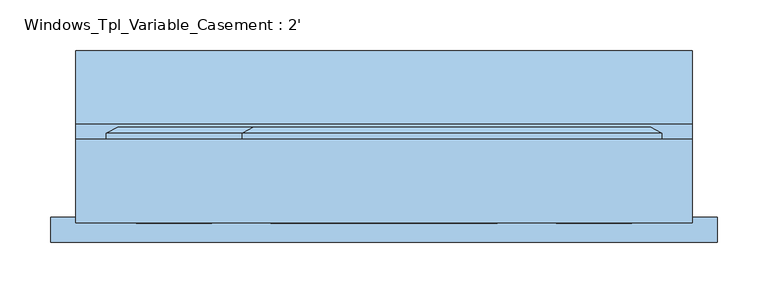
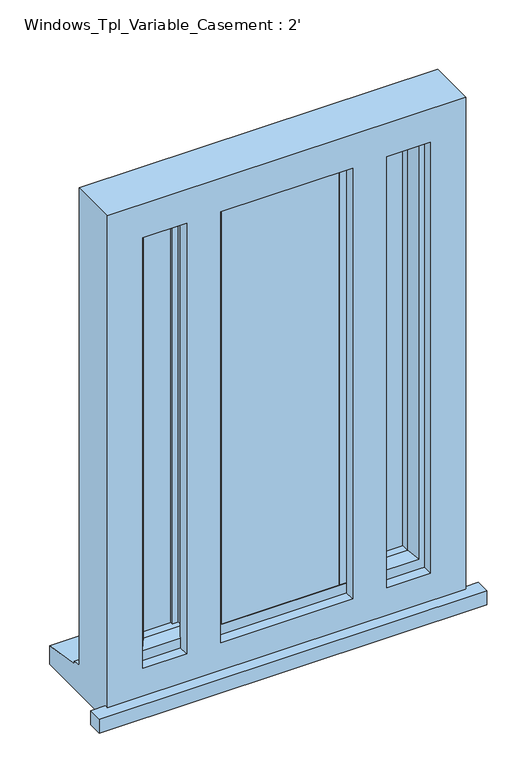
"""IFC4 building model written with IfcOpenShell, lengths in millimetres: window geometry, Windows_Tpl_Variable_Casement : 2'."""

from ifc_helpers import new_model, si_unit, frame, origin, place, context, project, spatial, polyline, outline, extrude, faceted_brep, source, transform, mapped, element, save


def windows_tpl_variable_casement_2_4efd9f92(model_context):
    return source(origin(), model_context, "Body", "SolidModel", [
        extrude(outline(polyline([(-319.6, -80.0942322), (-319.6, -55.0942322), (-294.6, -55.0942322), (-294.6, -60.9926322), (315.0, -60.9926322), (315.0, -55.0942322), (340.0, -55.0942322), (340.0, -80.0942322), (-319.6, -80.0942322)])), frame((0.0, 0.0, 1200.0), z_axis=(0.0, 0.0, 1.0), x_axis=(1.0, 0.0, 0.0)), (0.0, 0.0, 1.0), 25.0),
        faceted_brep([(-130.0, 22.0073678, 2080.0), (-130.0, 27.7808705, 2080.0), (-130.0, 27.7808705, 1253.0), (-130.0, 22.0073678, 1253.0), (-120.0, -42.9926322, 2070.0), (-120.0, 22.0073678, 2070.0), (-120.0, 22.0073678, 1263.0), (-120.0, -42.9926322, 1263.0), (-80.0, -28.4997323, 2030.0), (-90.1480377, -42.9926322, 2040.1480377), (-90.1480377, -42.9926322, 1292.8519623), (-80.0, -28.4997323, 1303.0), (-80.0, -13.9926322, 2030.0), (-80.0, -13.9926322, 1303.0), (-90.0, 10.0073678, 2040.0), (-90.0, -13.9926322, 2040.0), (-90.0, -13.9926322, 1293.0), (-90.0, 10.0073678, 1293.0), (-80.0, 27.7808705, 2030.0), (-80.0, 10.0073678, 2030.0), (-80.0, 10.0073678, 1303.0), (-80.0, 27.7808705, 1303.0), (-97.4457548, 33.5543732, 2047.4457548), (-97.4457548, 33.5543732, 1285.5542452), (-119.2153903, 33.5543732, 2069.2153903), (-119.2153903, 33.5543732, 1263.7846097), (285.0, 27.7808705, 1253.0), (285.0, 22.0073678, 1253.0), (275.0, 22.0073678, 1263.0), (275.0, -42.9926322, 1263.0), (245.1480377, -42.9926322, 1292.8519623), (235.0, -28.4997323, 1303.0), (235.0, -13.9926322, 1303.0), (245.0, -13.9926322, 1293.0), (245.0, 10.0073678, 1293.0), (235.0, 10.0073678, 1303.0), (235.0, 27.7808705, 1303.0), (252.4457548, 33.5543732, 1285.5542452), (274.2153903, 33.5543732, 1263.7846097), (285.0, 27.7808705, 2080.0), (285.0, 22.0073678, 2080.0), (275.0, 22.0073678, 2070.0), (275.0, -42.9926322, 2070.0), (245.1480377, -42.9926322, 2040.1480377), (235.0, -28.4997323, 2030.0), (235.0, -13.9926322, 2030.0), (245.0, -13.9926322, 2040.0), (245.0, 10.0073678, 2040.0), (235.0, 10.0073678, 2030.0), (235.0, 27.7808705, 2030.0), (252.4457548, 33.5543732, 2047.4457548), (274.2153903, 33.5543732, 2069.2153903)], [[[0, 1, 2, 3]], [[4, 5, 6, 7]], [[8, 9, 10, 11]], [[12, 8, 11, 13]], [[14, 15, 16, 17]], [[18, 19, 20, 21]], [[22, 18, 21, 23]], [[1, 24, 25, 2]], [[3, 2, 26, 27]], [[7, 6, 28, 29]], [[11, 10, 30, 31]], [[13, 11, 31, 32]], [[17, 16, 33, 34]], [[21, 20, 35, 36]], [[23, 21, 36, 37]], [[2, 25, 38, 26]], [[27, 26, 39, 40]], [[29, 28, 41, 42]], [[31, 30, 43, 44]], [[32, 31, 44, 45]], [[34, 33, 46, 47]], [[36, 35, 48, 49]], [[37, 36, 49, 50]], [[26, 38, 51, 39]], [[40, 39, 1, 0]], [[3, 27, 40, 0], [5, 41, 28, 6]], [[42, 41, 5, 4]], [[7, 29, 42, 4], [9, 43, 30, 10]], [[44, 43, 9, 8]], [[45, 44, 8, 12]], [[15, 46, 33, 16], [13, 32, 45, 12]], [[47, 46, 15, 14]], [[17, 34, 47, 14], [19, 48, 35, 20]], [[49, 48, 19, 18]], [[50, 49, 18, 22]], [[24, 51, 38, 25], [23, 37, 50, 22]], [[39, 51, 24, 1]]]),
        faceted_brep([(150.4, 22.0073678, 2080.0), (150.4, 27.7808705, 2080.0), (-264.6, 27.7808705, 2080.0), (-264.6, 22.0073678, 2080.0), (140.4, -42.9926322, 2070.0), (140.4, 22.0073678, 2070.0), (-254.6, 22.0073678, 2070.0), (-254.6, -42.9926322, 2070.0), (100.4, -28.4997323, 2030.0), (110.5480377, -42.9926322, 2040.1480377), (-224.7480377, -42.9926322, 2040.1480377), (-214.6, -28.4997323, 2030.0), (100.4, -13.9926322, 2030.0), (-214.6, -13.9926322, 2030.0), (110.4, 10.0073678, 2040.0), (110.4, -13.9926322, 2040.0), (-224.6, -13.9926322, 2040.0), (-224.6, 10.0073678, 2040.0), (100.4, 27.7808705, 2030.0), (100.4, 10.0073678, 2030.0), (-214.6, 10.0073678, 2030.0), (-214.6, 27.7808705, 2030.0), (119.2145656, 33.5543732, 2048.8145656), (-233.4145656, 33.5543732, 2048.8145656), (138.7692194, 33.5543732, 2068.3692194), (-252.9692194, 33.5543732, 2068.3692194), (-264.6, 27.7808705, 1253.0), (-264.6, 22.0073678, 1253.0), (-254.6, 22.0073678, 1263.0), (-254.6, -42.9926322, 1263.0), (-224.7480377, -42.9926322, 1292.8519623), (-214.6, -28.4997323, 1303.0), (-214.6, -13.9926322, 1303.0), (-224.6, -13.9926322, 1293.0), (-224.6, 10.0073678, 1293.0), (-214.6, 10.0073678, 1303.0), (-214.6, 27.7808705, 1303.0), (-233.4145656, 33.5543732, 1284.1854344), (-252.9692194, 33.5543732, 1264.6307806), (150.4, 27.7808705, 1253.0), (150.4, 22.0073678, 1253.0), (140.4, 22.0073678, 1263.0), (140.4, -42.9926322, 1263.0), (110.5480377, -42.9926322, 1292.8519623), (100.4, -28.4997323, 1303.0), (100.4, -13.9926322, 1303.0), (110.4, -13.9926322, 1293.0), (110.4, 10.0073678, 1293.0), (100.4, 10.0073678, 1303.0), (100.4, 27.7808705, 1303.0), (119.2145656, 33.5543732, 1284.1854344), (138.7692194, 33.5543732, 1264.6307806)], [[[0, 1, 2, 3]], [[4, 5, 6, 7]], [[8, 9, 10, 11]], [[12, 8, 11, 13]], [[14, 15, 16, 17]], [[18, 19, 20, 21]], [[22, 18, 21, 23]], [[1, 24, 25, 2]], [[3, 2, 26, 27]], [[7, 6, 28, 29]], [[11, 10, 30, 31]], [[13, 11, 31, 32]], [[17, 16, 33, 34]], [[21, 20, 35, 36]], [[23, 21, 36, 37]], [[2, 25, 38, 26]], [[27, 26, 39, 40]], [[0, 3, 27, 40], [41, 28, 6, 5]], [[29, 28, 41, 42]], [[4, 7, 29, 42], [43, 30, 10, 9]], [[31, 30, 43, 44]], [[32, 31, 44, 45]], [[46, 33, 16, 15], [12, 13, 32, 45]], [[34, 33, 46, 47]], [[14, 17, 34, 47], [48, 35, 20, 19]], [[36, 35, 48, 49]], [[37, 36, 49, 50]], [[51, 38, 25, 24], [22, 23, 37, 50]], [[26, 38, 51, 39]], [[40, 39, 1, 0]], [[42, 41, 5, 4]], [[44, 43, 9, 8]], [[45, 44, 8, 12]], [[47, 46, 15, 14]], [[49, 48, 19, 18]], [[50, 49, 18, 22]], [[39, 51, 24, 1]]]),
        faceted_brep([(315.0, -60.9926322, 2110.0), (-294.6, -60.9926322, 2110.0), (-294.6, -60.9926322, 1200.0), (315.0, -60.9926322, 1200.0), (255.0, -60.9926322, 2050.0), (255.0, -60.9926322, 1275.0), (180.4, -60.9926322, 1275.0), (180.4, -60.9926322, 2050.0), (-160.0, -60.9926322, 2050.0), (-160.0, -60.9926322, 1275.0), (-234.6, -60.9926322, 1275.0), (-234.6, -60.9926322, 2050.0), (122.4, -60.9926322, 2050.0), (122.4, -60.9926322, 1275.0), (-102.0, -60.9926322, 1275.0), (-102.0, -60.9926322, 2050.0), (-294.6, 22.0073678, 2110.0), (-294.6, 22.0073678, 1251.0), (-294.6, 37.0073678, 1249.68767), (-294.6, 37.0073678, 1244.7449676), (-294.6, 109.5073678, 1233.8088847), (-294.6, 109.5073678, 1200.0), (315.0, 22.0073678, 2110.0), (315.0, 22.0073678, 1251.0), (-254.6, 22.0073678, 2070.0), (-254.6, 22.0073678, 1263.0), (-160.0, 22.0073678, 1263.0), (-160.0, 22.0073678, 2070.0), (180.4, 22.0073678, 2070.0), (180.4, 22.0073678, 1263.0), (275.0, 22.0073678, 1263.0), (275.0, 22.0073678, 2070.0), (-120.0, 22.0073678, 2070.0), (-120.0, 22.0073678, 1263.0), (140.4, 22.0073678, 1263.0), (140.4, 22.0073678, 2070.0), (-254.6, -42.9926322, 2070.0), (-254.6, -42.9926322, 1263.0), (-150.0, -42.9926322, 2070.0), (-150.0, -42.9926322, 1263.0), (-160.0, -42.9926322, 2050.0), (-234.6, -42.9926322, 2050.0), (-234.6, -42.9926322, 1275.0), (-160.0, -42.9926322, 1275.0), (-120.0, -42.9926322, 2070.0), (140.4, -42.9926322, 2070.0), (140.4, -42.9926322, 1263.0), (-120.0, -42.9926322, 1263.0), (122.4, -42.9926322, 2050.0), (-102.0, -42.9926322, 2050.0), (-102.0, -42.9926322, 1275.0), (122.4, -42.9926322, 1275.0), (170.4, -42.9926322, 2070.0), (275.0, -42.9926322, 2070.0), (275.0, -42.9926322, 1263.0), (170.4, -42.9926322, 1263.0), (255.0, -42.9926322, 2050.0), (180.4, -42.9926322, 2050.0), (180.4, -42.9926322, 1275.0), (255.0, -42.9926322, 1275.0), (-160.0, -18.9926322, 2070.0), (-150.0, -18.9926322, 2070.0), (170.4, -18.9926322, 2070.0), (180.4, -18.9926322, 2070.0), (315.0, 109.5073678, 1200.0), (315.0, 109.5073678, 1233.8088847), (315.0, 37.0073678, 1244.7449676), (315.0, 37.0073678, 1249.68767), (180.4, -18.9926322, 1263.0), (170.4, -18.9926322, 1263.0), (-150.0, -18.9926322, 1263.0), (-160.0, -18.9926322, 1263.0)], [[[0, 1, 2, 3], [4, 5, 6, 7], [8, 9, 10, 11], [12, 13, 14, 15]], [[2, 1, 16, 17, 18, 19, 20, 21]], [[17, 16, 22, 23], [24, 25, 26, 27], [28, 29, 30, 31], [32, 33, 34, 35]], [[25, 24, 36, 37]], [[36, 38, 39, 37], [40, 41, 42, 43]], [[44, 45, 46, 47], [48, 49, 50, 51]], [[52, 53, 54, 55], [56, 57, 58, 59]], [[41, 11, 10, 42]], [[1, 0, 22, 16]], [[36, 24, 27, 60, 61, 38]], [[35, 45, 44, 32]], [[31, 53, 52, 62, 63, 28]], [[11, 41, 40, 8]], [[48, 12, 15, 49]], [[56, 4, 7, 57]], [[23, 22, 0, 3, 64, 65, 66, 67]], [[31, 30, 54, 53]], [[4, 56, 59, 5]], [[57, 7, 6, 58]], [[12, 48, 51, 13]], [[35, 34, 46, 45]], [[29, 28, 63, 68]], [[68, 63, 62, 69]], [[69, 62, 52, 55]], [[61, 70, 39, 38]], [[70, 61, 60, 71]], [[71, 60, 27, 26]], [[33, 32, 44, 47]], [[49, 15, 14, 50]], [[8, 40, 43, 9]], [[64, 3, 2, 21]], [[65, 64, 21, 20]], [[66, 65, 20, 19]], [[67, 66, 19, 18]], [[23, 67, 18, 17]], [[26, 25, 37, 39, 70, 71]], [[34, 33, 47, 46]], [[55, 54, 30, 29, 68, 69]], [[6, 5, 59, 58]], [[14, 13, 51, 50]], [[43, 42, 10, 9]]]),
        extrude(outline(polyline([(110.4, -13.9926322), (-224.6, -13.9926322), (-224.6, 10.0073678), (110.4, 10.0073678), (110.4, -13.9926322)])), frame((0.0, 0.0, 1293.0), z_axis=(0.0, 0.0, 1.0), x_axis=(1.0, 0.0, 0.0)), (0.0, 0.0, 1.0), 747.0),
        extrude(outline(polyline([(-150.0, -18.9926322), (170.4, -18.9926322), (170.4, -42.9926322), (-150.0, -42.9926322), (-150.0, -18.9926322)])), frame((0.0, 0.0, 1263.0), z_axis=(0.0, 0.0, 1.0), x_axis=(1.0, 0.0, 0.0)), (0.0, 0.0, 1.0), 807.0),
        extrude(outline(polyline([(245.0, -13.9926322), (-90.0, -13.9926322), (-90.0, 10.0073678), (245.0, 10.0073678), (245.0, -13.9926322)])), frame((0.0, 0.0, 1293.0), z_axis=(0.0, 0.0, 1.0), x_axis=(1.0, 0.0, 0.0)), (0.0, 0.0, 1.0), 747.0),
    ])


if __name__ == "__main__":
    model = new_model("IFC4")
    model_context = context("Model", 3, world=origin())
    ifc_project = project(units=[si_unit("LENGTHUNIT", "METRE", prefix="MILLI")], contexts=[model_context])
    site = spatial("IfcSite", under=ifc_project)
    building = spatial("IfcBuilding", under=site)
    placement = place(None, origin())
    windows_tpl_variable_casement_2_shape = windows_tpl_variable_casement_2_4efd9f92(model_context)
    element("IfcWindow", 1, ObjectType="Windows_Tpl_Variable_Casement : 2'", at=placement, inside=building, context=model_context, shape_type="MappedRepresentation", body=[
        mapped(windows_tpl_variable_casement_2_shape, transform((0.0, 0.0, 0.0), x_axis=(1.0, 0.0, 0.0), y_axis=(0.0, 1.0, 0.0), z_axis=(0.0, 0.0, 1.0))),
    ])
    save(model, "model.ifc")

# Revit data of these elements
# Type "Windows_Tpl_Variable_Casement : 2'"
#   Type Mark = "82"
#   Operation = "TriplePanelVertical"
#   Construction Type Id = "GSP4R"
#   Manufacturer = "Revit"
#   Keynote = "L10"
#   Analytic Construction = "1/8 in Pilkington single glazing"
#   Wrap Layers (Int) from Ext = 177.5 mm
#   Wrap Layers (Ext) from Ext = 102.5 mm
#   Window Board Projection = 25 mm
#   Window Board Extension = 25 mm
#   Visual Light Transmittance = 0.9
#   Solar Heat Gain Coefficient = 0.78
#   Rough Width = 609.6 mm
#   Rough Height = 910 mm
#   Height = 910 mm
#   Width = 609.6 mm
#   Heat Transfer Coefficient (U) = 3.6886 W/(m²·K)
#   Glazing Thickness = 24 mm
#   FrameOffset - External = 50 mm
#   Frame Depth = 65 mm
#   Default Head Height = 2110 mm
#   Cill Depth = 87.5 mm
#   Cavity Closer Width = 50 mm
#   Cavity Closer Offset from Ext = 102.5 mm
#   Cavity Closer Depth = 85 mm
#   Casement Width = 450 mm
#   Vis - Cavity Closers = yes
#   Define Thermal Properties by = 1
#   Material Trim = Window Frame
#   Material Glass = Glass
#   Material Frame = Window Frame
#   Wall Closure = (empty or 0)
# Element 1 (IfcWindow, "Windows_Tpl_Variable_Casement : 2'")
#   Materials on its faces: "Window Frame", "Glass"
# Materials
#   "Window Frame": colour RGB 249 249 249, transparency 0, Keynote = "L10", Cost = 0
#   "Glass": class "Glass", colour RGB 0 128 192, transparency 0.9, Description = "Soda Lime Glass", Cost = 0
